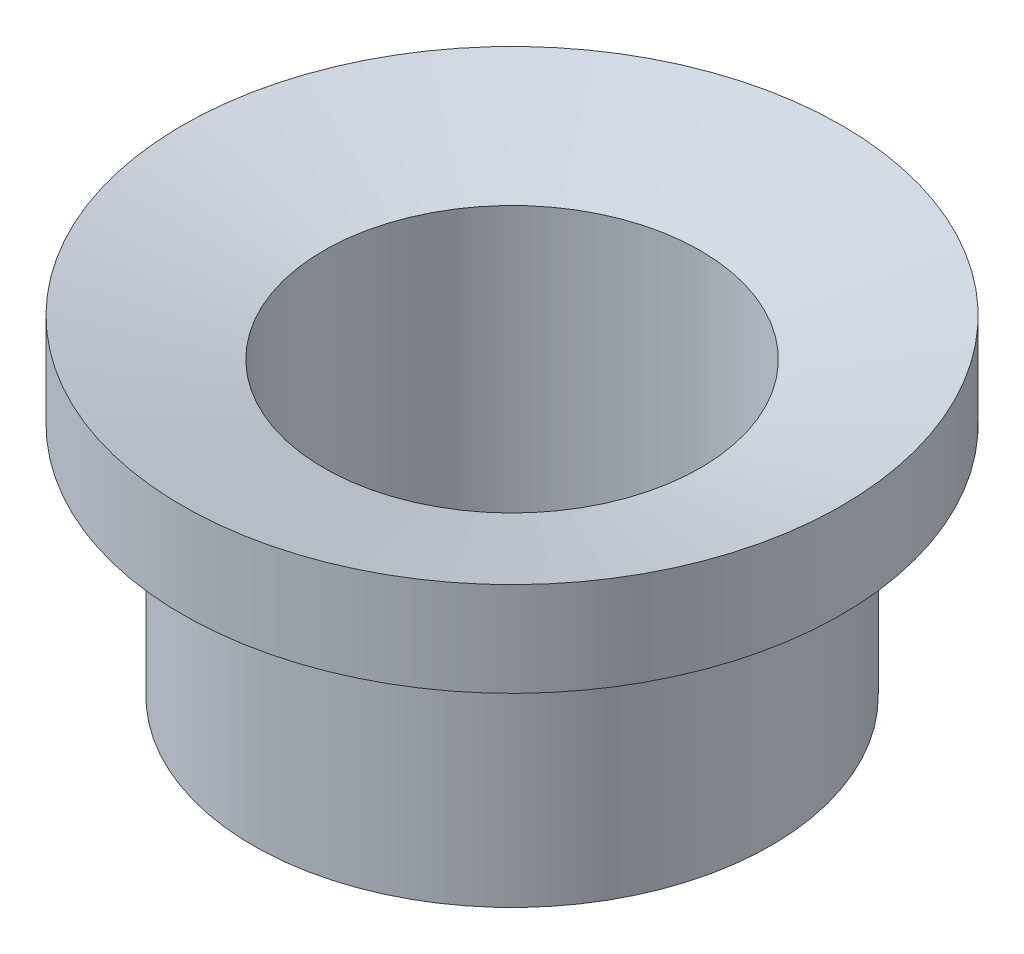
SolidWorks part; units mm, degrees
material "Brass"
ref_plane "Front Plane" through (0, 0, 0) normal (0, 0, 1) x (1, 0, 0)
ref_plane "Top Plane" through (0, 0, 0) normal (0, 1, 0) x (1, 0, 0)
ref_plane "Right Plane" through (0, 0, 0) normal (1, 0, 0) x (0, 0, -1)
sketch "Bush Profile Sketch" plane through (0, 0, 0) normal (0, 0, 1) x (1, 0, 0)
  line L0 (0, -13.8696) -> (0, 22.4783) construction
  line L1 (-12, 0) -> (-12, 18.5885)
  line L2 (-12, 18.5885) -> (-21, 21)
  line L3 (-21, 21) -> (-21, 15)
  line L4 (-21, 15) -> (-16.5, 15)
  line L5 (-16.5, 15) -> (-16.5, 0)
  line L6 (-16.5, 0) -> (-12, 0)
  line L7 (-21, 21) -> (-7.9565, 21) construction
  dimension "D1" = 6
  dimension "D2" = 15
  dimension "D3" = 16.5
  dimension "D4" = 12
  dimension "D5" = 21
  dimension "D6" = 15
revolve "Flanged Bush Revolve" add sketch "Bush Profile Sketch" angle 360 about L0
